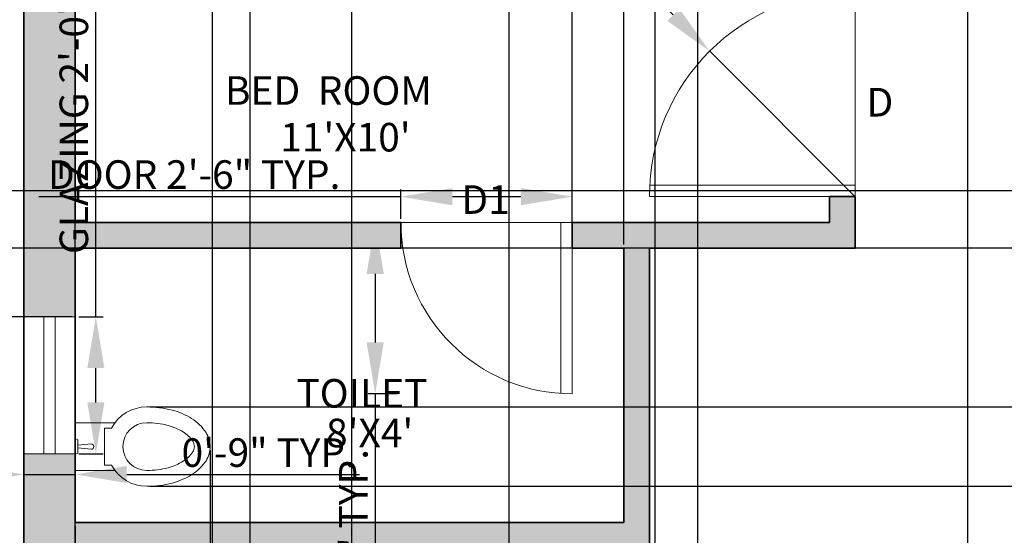
# Model space of a CAD drawing. Units: inches. Extents: x 2265 to 2807, y 1544 to 2401.
# Tile 4 of 9: x 2358 to 2531, y 2073 to 2164. Entities that reach past the tile are written whole.
import ezdxf

# ---------------------------------------------------------------- set-up
doc = ezdxf.new("R2010")
doc.units = ezdxf.units.IN
for name, color, linetype, lineweight in [('A-ANNO-DIMS', 2, 'Continuous', 18), ('A-ANNO-TEXT', 7, 'Continuous', 18), ('A-AREA-IDEN', 7, 'Continuous', 18), ('A-DOOR', 3, 'Continuous', 18), ('A-FLOR-FIXT', 8, 'Continuous', 18), ('A-GLAZ', 4, 'Continuous', 18), ('A-WALL', 7, 'Continuous', 35), ('A-WALL-PATT', 18, 'Continuous', 13)]:
    doc.layers.add(name, color=color, linetype=linetype, lineweight=lineweight)
doc.styles.add('ARIAL', font='times.ttf', dxfattribs={"height": 5})
doc.styles.get("Standard").update_dxf_attribs({"font": 'arial.ttf', "height": 5})
doc.dimstyles.new('ISO-25', dxfattribs={"dimtxt": 5, "dimasz": 9, "dimexe": 1.25, "dimexo": 0.625, "dimtad": 1, "dimlunit": 3, "dimtxsty": 'Standard', "dimcen": 2.5, "dimadec": 0, "dimazin": 0, "dimtfac": 1, "dimtmove": 0, "dimatfit": 3, "dimfxl": 1, "dimarcsym": 0})

# ---------------------------------------------------------------- blocks, each defined once
blk = doc.blocks.new('GLAZING-24IN')
for p, q in [((0, 24), (0, 0)), ((3.5, 24), (3.5, 0)), ((5.5, 24), (5.5, 0)), ((5.5, 24), (5.5, 0)), ((9, 0), (9, 24))]:
    blk.add_line(p, q)
blk = doc.blocks.new('DOOR-SWING-30IN')
for p, q in [((2, 29.93), (2, 0)), ((0, 0), (30, 0))]:
    blk.add_line(p, q)
blk.add_arc((0, 0), 30, 0, 90)
blk = doc.blocks.new('*D17')
at = {"layer": 'A-ANNO-DIMS', "color": 0, "lineweight": -2, "transparency": 16777216}
for p, q in [((2353.7, 2031.88), (2353.7, 2105.4)), ((2358.48, 2031.88), (2352.45, 2031.88)), ((2353.7, 2004.88), (2353.7, 2022.88)), ((2358.48, 1995.88), (2352.45, 1995.88))]:
    blk.add_line(p, q, dxfattribs=at)
at = {"layer": 'A-ANNO-DIMS', "color": 0, "lineweight": 100, "transparency": 16777216}
for points in [[(2352.2, 2022.88), (2355.2, 2022.88), (2353.7, 2031.88)], [(2352.2, 2004.88), (2355.2, 2004.88), (2353.7, 1995.88)]]:
    blk.add_solid(points, dxfattribs=at)
at = {"layer": 'Defpoints', "color": 0, "lineweight": 100, "transparency": 16777216}
for p in [(2353.7, 2031.88), (2359.1, 2031.88), (2359.1, 1995.88)]:
    blk.add_point(p, dxfattribs=at)
at = {"layer": 'A-ANNO-DIMS', "color": 0, "transparency": 16777216, "insert": (2350.49, 2073.14), "char_height": 5, "attachment_point": 5, "rotation": 90}
blk.add_mtext('WINDOW 3\'-0" TYP.', dxfattribs=at)
blk = doc.blocks.new('*D21')
at = {"layer": 'A-ANNO-DIMS', "color": 0, "lineweight": -2, "transparency": 16777216}
for p, q in [((2371.7, 2111.73), (2371.7, 2184.98)), ((2368.73, 2111.73), (2372.95, 2111.73)), ((2371.7, 2096.73), (2371.7, 2102.73)), ((2368.73, 2087.73), (2372.95, 2087.73))]:
    blk.add_line(p, q, dxfattribs=at)
at = {"layer": 'A-ANNO-DIMS', "color": 0, "lineweight": 100, "transparency": 16777216}
for points in [[(2370.2, 2102.73), (2373.2, 2102.73), (2371.7, 2111.73)], [(2370.2, 2096.73), (2373.2, 2096.73), (2371.7, 2087.73)]]:
    blk.add_solid(points, dxfattribs=at)
at = {"layer": 'Defpoints', "color": 0, "lineweight": 100, "transparency": 16777216}
for p in [(2368.1, 2111.73), (2371.7, 2111.73), (2368.1, 2087.73)]:
    blk.add_point(p, dxfattribs=at)
at = {"layer": 'A-ANNO-DIMS', "color": 0, "transparency": 16777216, "insert": (2368.49, 2152.86), "char_height": 5, "attachment_point": 5, "rotation": 90}
blk.add_mtext('GLAZING 2\'-0" TYP.', dxfattribs=at)
blk = doc.blocks.new('*D22')
at = {"layer": 'A-ANNO-DIMS', "color": 0, "lineweight": -2, "transparency": 16777216}
for p, q in [((2359.1, 2087.11), (2359.1, 2082.88)), ((2368.1, 2087.11), (2368.1, 2082.88)), ((2350.1, 2084.13), (2341.1, 2084.13)), ((2359.1, 2084.13), (2368.1, 2084.13)), ((2377.1, 2084.13), (2417.83, 2084.13))]:
    blk.add_line(p, q, dxfattribs=at)
at = {"layer": 'A-ANNO-DIMS', "color": 0, "lineweight": 100, "transparency": 16777216}
for points in [[(2350.1, 2085.63), (2350.1, 2082.63), (2359.1, 2084.13)], [(2377.1, 2085.63), (2377.1, 2082.63), (2368.1, 2084.13)]]:
    blk.add_solid(points, dxfattribs=at)
at = {"layer": 'Defpoints', "color": 0, "lineweight": 100, "transparency": 16777216}
for p in [(2359.1, 2087.73), (2368.1, 2087.73), (2368.1, 2084.13)]:
    blk.add_point(p, dxfattribs=at)
at = {"layer": 'A-ANNO-DIMS', "color": 0, "transparency": 16777216, "insert": (2401.96, 2087.31), "char_height": 5, "attachment_point": 5}
blk.add_mtext('0\'-9" TYP.', dxfattribs=at)
blk = doc.blocks.new('*D23')
at = {"layer": 'A-ANNO-DIMS', "color": 0, "lineweight": -2, "transparency": 16777216}
for p, q in [((2425.1, 2128.86), (2425.1, 2133.98)), ((2455.1, 2128.86), (2455.1, 2133.98)), ((2425.1, 2132.73), (2361.73, 2132.73)), ((2446.1, 2132.73), (2434.1, 2132.73))]:
    blk.add_line(p, q, dxfattribs=at)
at = {"layer": 'A-ANNO-DIMS', "color": 0, "lineweight": 100, "transparency": 16777216}
for points in [[(2434.1, 2134.23), (2434.1, 2131.23), (2425.1, 2132.73)], [(2446.1, 2134.23), (2446.1, 2131.23), (2455.1, 2132.73)]]:
    blk.add_solid(points, dxfattribs=at)
at = {"layer": 'Defpoints', "color": 0, "lineweight": 100, "transparency": 16777216}
for p in [(2425.1, 2132.73), (2425.1, 2128.23), (2455.1, 2128.23)]:
    blk.add_point(p, dxfattribs=at)
at = {"layer": 'A-ANNO-DIMS', "color": 0, "transparency": 16777216, "insert": (2388.91, 2135.95), "char_height": 5, "attachment_point": 5}
blk.add_mtext('DOOR 2\'-6" TYP.', dxfattribs=at)
blk = doc.blocks.new('*D24')
at = {"layer": 'A-ANNO-DIMS', "color": 0, "lineweight": -2, "transparency": 16777216}
for p, q in [((2424.48, 2128.23), (2419.35, 2128.23)), ((2420.6, 2119.23), (2420.6, 2107.23)), ((2424.48, 2098.23), (2419.35, 2098.23)), ((2420.6, 2098.23), (2420.6, 2057.42))]:
    blk.add_line(p, q, dxfattribs=at)
at = {"layer": 'A-ANNO-DIMS', "color": 0, "lineweight": 100, "transparency": 16777216}
for points in [[(2419.1, 2119.23), (2422.1, 2119.23), (2420.6, 2128.23)], [(2419.1, 2107.23), (2422.1, 2107.23), (2420.6, 2098.23)]]:
    blk.add_solid(points, dxfattribs=at)
at = {"layer": 'Defpoints', "color": 0, "lineweight": 100, "transparency": 16777216}
for p in [(2425.1, 2128.23), (2420.6, 2098.23), (2425.1, 2098.23)]:
    blk.add_point(p, dxfattribs=at)
at = {"layer": 'A-ANNO-DIMS', "color": 0, "transparency": 16777216, "insert": (2417.42, 2073.33), "char_height": 5, "attachment_point": 5, "rotation": 90}
blk.add_mtext('2\'-6" TYP.', dxfattribs=at)
blk = doc.blocks.new('*D40')
at = {"layer": 'A-ANNO-DIMS', "color": 0, "lineweight": -2, "transparency": 16777216}
for p, q in [((2368.1, 2005.86), (2368.1, 2297.59)), ((2392.1, 2005.86), (2392.1, 2297.59)), ((2377.1, 2296.34), (2383.1, 2296.34))]:
    blk.add_line(p, q, dxfattribs=at)
at = {"layer": 'A-ANNO-DIMS', "color": 0, "lineweight": 100, "transparency": 16777216}
for points in [[(2377.1, 2297.84), (2377.1, 2294.84), (2368.1, 2296.34)], [(2383.1, 2297.84), (2383.1, 2294.84), (2392.1, 2296.34)]]:
    blk.add_solid(points, dxfattribs=at)
at = {"layer": 'Defpoints', "color": 0, "lineweight": 100, "transparency": 16777216}
for p in [(2392.1, 2296.34), (2368.1, 2005.23), (2392.1, 2005.23)]:
    blk.add_point(p, dxfattribs=at)
at = {"layer": 'A-ANNO-DIMS', "color": 0, "transparency": 16777216, "insert": (2380.1, 2299.52), "char_height": 5, "attachment_point": 5}
blk.add_mtext('2\'-0"', dxfattribs=at)
blk = doc.blocks.new('*D43')
at = {"layer": 'A-ANNO-DIMS', "color": 0, "lineweight": -2, "transparency": 16777216}
for p, q in [((2416.49, 1959.08), (2416.49, 2297.59)), ((2444.05, 1959.08), (2444.05, 2297.59)), ((2425.49, 2296.34), (2435.05, 2296.34))]:
    blk.add_line(p, q, dxfattribs=at)
at = {"layer": 'A-ANNO-DIMS', "color": 0, "lineweight": 100, "transparency": 16777216}
for points in [[(2425.49, 2297.84), (2425.49, 2294.84), (2416.49, 2296.34)], [(2435.05, 2297.84), (2435.05, 2294.84), (2444.05, 2296.34)]]:
    blk.add_solid(points, dxfattribs=at)
at = {"layer": 'Defpoints', "color": 0, "lineweight": 100, "transparency": 16777216}
for p in [(2444.05, 2296.34), (2416.49, 1958.45), (2444.05, 1958.45)]:
    blk.add_point(p, dxfattribs=at)
at = {"layer": 'A-ANNO-DIMS', "color": 0, "transparency": 16777216, "insert": (2430.27, 2299.56), "char_height": 5, "attachment_point": 5}
blk.add_mtext('2\'-3 1/2"', dxfattribs=at)
blk = doc.blocks.new('*D45')
at = {"layer": 'A-ANNO-DIMS', "color": 0, "lineweight": -2, "transparency": 16777216}
for p, q in [((2391.72, 2088.38), (2391.72, 1546.93)), ((2368.1, 2075.11), (2368.1, 1546.93)), ((2377.1, 1548.18), (2382.72, 1548.18)), ((2391.72, 1548.18), (2430.33, 1548.18))]:
    blk.add_line(p, q, dxfattribs=at)
at = {"layer": 'A-ANNO-DIMS', "color": 0, "lineweight": 100, "transparency": 16777216}
for points in [[(2377.1, 1549.68), (2377.1, 1546.68), (2368.1, 1548.18)], [(2382.72, 1549.68), (2382.72, 1546.68), (2391.72, 1548.18)]]:
    blk.add_solid(points, dxfattribs=at)
at = {"layer": 'Defpoints', "color": 0, "lineweight": 100, "transparency": 16777216}
for p in [(2391.72, 2089), (2368.1, 2075.73), (2391.72, 1548.18)]:
    blk.add_point(p, dxfattribs=at)
at = {"layer": 'A-ANNO-DIMS', "color": 0, "transparency": 16777216, "insert": (2415.53, 1551.4), "char_height": 5, "attachment_point": 5}
blk.add_mtext('1\'-11 1/2"', dxfattribs=at)
blk = doc.blocks.new('*D46')
at = {"layer": 'A-ANNO-DIMS', "color": 0, "lineweight": -2, "transparency": 16777216}
for p, q in [((2803.21, 2104.95), (2803.21, 2128.02)), ((2381.23, 2095.95), (2804.46, 2095.95)), ((2803.21, 2082.06), (2803.21, 2095.95)), ((2381.23, 2082.06), (2804.46, 2082.06)), ((2803.21, 2073.06), (2803.21, 2064.06))]:
    blk.add_line(p, q, dxfattribs=at)
at = {"layer": 'A-ANNO-DIMS', "color": 0, "lineweight": 100, "transparency": 16777216}
for points in [[(2801.71, 2104.95), (2804.71, 2104.95), (2803.21, 2095.95)], [(2801.71, 2073.06), (2804.71, 2073.06), (2803.21, 2082.06)]]:
    blk.add_solid(points, dxfattribs=at)
at = {"layer": 'Defpoints', "color": 0, "lineweight": 100, "transparency": 16777216}
for p in [(2380.61, 2095.95), (2803.21, 2095.95), (2380.61, 2082.06)]:
    blk.add_point(p, dxfattribs=at)
at = {"layer": 'A-ANNO-DIMS', "color": 0, "transparency": 16777216, "insert": (2800.07, 2120.99), "char_height": 5, "attachment_point": 5, "rotation": 90}
blk.add_mtext('1\'-2"', dxfattribs=at)
blk = doc.blocks.new('*D47')
at = {"layer": 'A-ANNO-DIMS', "color": 0, "lineweight": -2, "transparency": 16777216}
for p, q in [((2455.1, 2124.36), (2455.1, 2297.59)), ((2464.1, 2124.36), (2464.1, 2297.59)), ((2446.1, 2296.34), (2437.1, 2296.34)), ((2455.1, 2296.34), (2464.1, 2296.34)), ((2473.1, 2296.34), (2496.64, 2296.34))]:
    blk.add_line(p, q, dxfattribs=at)
at = {"layer": 'A-ANNO-DIMS', "color": 0, "lineweight": 100, "transparency": 16777216}
for points in [[(2446.1, 2297.84), (2446.1, 2294.84), (2455.1, 2296.34)], [(2473.1, 2297.84), (2473.1, 2294.84), (2464.1, 2296.34)]]:
    blk.add_solid(points, dxfattribs=at)
at = {"layer": 'Defpoints', "color": 0, "lineweight": 100, "transparency": 16777216}
for p in [(2464.1, 2296.34), (2455.1, 2123.73), (2464.1, 2123.73)]:
    blk.add_point(p, dxfattribs=at)
at = {"layer": 'A-ANNO-DIMS', "color": 0, "transparency": 16777216, "insert": (2489.37, 2299.52), "char_height": 5, "attachment_point": 5}
blk.add_mtext('0\'-9"', dxfattribs=at)
blk = doc.blocks.new('*D49')
at = {"layer": 'A-ANNO-DIMS', "color": 0, "lineweight": -2, "transparency": 16777216}
for p, q in [((2275.29, 2132.73), (2275.29, 2155.8)), ((2367.48, 2123.73), (2274.04, 2123.73)), ((2275.29, 2111.73), (2275.29, 2123.73)), ((2367.48, 2111.73), (2274.04, 2111.73)), ((2275.29, 2102.73), (2275.29, 2093.73))]:
    blk.add_line(p, q, dxfattribs=at)
at = {"layer": 'A-ANNO-DIMS', "color": 0, "lineweight": 100, "transparency": 16777216}
for points in [[(2273.79, 2132.73), (2276.79, 2132.73), (2275.29, 2123.73)], [(2273.79, 2102.73), (2276.79, 2102.73), (2275.29, 2111.73)]]:
    blk.add_solid(points, dxfattribs=at)
at = {"layer": 'Defpoints', "color": 0, "lineweight": 100, "transparency": 16777216}
for p in [(2275.29, 2123.73), (2368.1, 2123.73), (2368.1, 2111.73)]:
    blk.add_point(p, dxfattribs=at)
at = {"layer": 'A-ANNO-DIMS', "color": 0, "transparency": 16777216, "insert": (2272.11, 2148.77), "char_height": 5, "attachment_point": 5, "rotation": 90}
blk.add_mtext('1\'-0"', dxfattribs=at)
blk = doc.blocks.new('*D50')
at = {"layer": 'A-ANNO-DIMS', "color": 0, "lineweight": -2, "transparency": 16777216}
for p, q in [((2398.67, 2169.19), (2398.67, 1546.93)), ((2469.53, 2169.19), (2469.53, 1546.93)), ((2407.67, 1548.18), (2460.53, 1548.18))]:
    blk.add_line(p, q, dxfattribs=at)
at = {"layer": 'A-ANNO-DIMS', "color": 0, "lineweight": 100, "transparency": 16777216}
for points in [[(2407.67, 1549.68), (2407.67, 1546.68), (2398.67, 1548.18)], [(2460.53, 1549.68), (2460.53, 1546.68), (2469.53, 1548.18)]]:
    blk.add_solid(points, dxfattribs=at)
at = {"layer": 'Defpoints', "color": 0, "lineweight": 100, "transparency": 16777216}
for p in [(2398.67, 2169.81), (2469.53, 2169.81), (2469.53, 1548.18)]:
    blk.add_point(p, dxfattribs=at)
at = {"layer": 'A-ANNO-DIMS', "color": 0, "transparency": 16777216, "insert": (2434.1, 1551.36), "char_height": 5, "attachment_point": 5}
blk.add_mtext('5\'-11"', dxfattribs=at)
blk = doc.blocks.new('*D60')
at = {"layer": 'A-ANNO-DIMS', "color": 0, "lineweight": -2, "transparency": 16777216}
for p, q in [((2275.29, 2142.73), (2275.29, 2151.73)), ((2580.48, 2133.73), (2274.04, 2133.73)), ((2275.29, 2133.73), (2275.29, 2123.73)), ((2580.48, 2123.73), (2274.04, 2123.73)), ((2275.29, 2114.73), (2275.29, 2087.31))]:
    blk.add_line(p, q, dxfattribs=at)
at = {"layer": 'A-ANNO-DIMS', "color": 0, "lineweight": 100, "transparency": 16777216}
for points in [[(2273.79, 2142.73), (2276.79, 2142.73), (2275.29, 2133.73)], [(2273.79, 2114.73), (2276.79, 2114.73), (2275.29, 2123.73)]]:
    blk.add_solid(points, dxfattribs=at)
at = {"layer": 'Defpoints', "color": 0, "lineweight": 100, "transparency": 16777216}
for p in [(2581.1, 2133.73), (2275.29, 2123.73), (2581.1, 2123.73)]:
    blk.add_point(p, dxfattribs=at)
at = {"layer": 'A-ANNO-DIMS', "color": 0, "transparency": 16777216, "insert": (2272.11, 2096.52), "char_height": 5, "attachment_point": 5, "rotation": 90}
blk.add_mtext('0\'-10"', dxfattribs=at)
blk = doc.blocks.new('*D63')
at = {"layer": 'A-ANNO-DIMS', "color": 0, "lineweight": -2, "transparency": 16777216}
for p, q in [((2477.1, 1993.66), (2477.1, 2297.59)), ((2524.34, 1993.66), (2524.34, 2297.59)), ((2486.1, 2296.34), (2515.34, 2296.34))]:
    blk.add_line(p, q, dxfattribs=at)
at = {"layer": 'A-ANNO-DIMS', "color": 0, "lineweight": 100, "transparency": 16777216}
for points in [[(2486.1, 2297.84), (2486.1, 2294.84), (2477.1, 2296.34)], [(2515.34, 2297.84), (2515.34, 2294.84), (2524.34, 2296.34)]]:
    blk.add_solid(points, dxfattribs=at)
at = {"layer": 'Defpoints', "color": 0, "lineweight": 100, "transparency": 16777216}
for p in [(2524.34, 2296.34), (2477.1, 1993.03), (2524.34, 1993.03)]:
    blk.add_point(p, dxfattribs=at)
at = {"layer": 'A-ANNO-DIMS', "color": 0, "transparency": 16777216, "insert": (2500.72, 2299.52), "char_height": 5, "attachment_point": 5}
blk.add_mtext('3\'-11"', dxfattribs=at)
blk = doc.blocks.new('*D66')
at = {"layer": 'A-ANNO-DIMS', "color": 0, "lineweight": -2, "transparency": 16777216}
for p, q in [((2452.75, 2184.58), (2472.78, 2164.55)), ((2504.6, 2132.73), (2479.15, 2158.19))]:
    blk.add_line(p, q, dxfattribs=at)
at = {"layer": 'A-ANNO-DIMS', "color": 0, "lineweight": 100, "transparency": 16777216}
blk.add_solid([(2473.84, 2165.61), (2471.72, 2163.49), (2479.15, 2158.19)], dxfattribs=at)
at = {"layer": 'Defpoints', "color": 0, "lineweight": 100, "transparency": 16777216}
for p in [(2479.15, 2158.19), (2504.6, 2132.73)]:
    blk.add_point(p, dxfattribs=at)
at = {"layer": 'A-ANNO-DIMS', "color": 0, "transparency": 16777216, "insert": (2461.83, 2180), "char_height": 5, "attachment_point": 5, "rotation": 315.0005}
blk.add_mtext('R3\'-0"', dxfattribs=at)

msp = doc.modelspace()

# ---------------------------------------------------------------- hatches: boundary and pattern name
at = {"layer": 'A-WALL-PATT'}
h = msp.add_hatch(color=256, dxfattribs=at)
h.dxf.hatch_style = 1
h.paths.add_polyline_path([(2416.101, 2255.733), (2359.101, 2255.733), (2359.101, 2205.483), (2368.101, 2205.483), (2368.101, 2246.733), (2416.101, 2246.733)])
h.paths.add_polyline_path([(2528.601, 2255.733), (2452.101, 2255.733), (2452.101, 2246.733), (2487.251, 2246.733), (2500.101, 2246.733), (2500.101, 2168.733), (2504.601, 2168.733), (2504.601, 2170.233), (2525.601, 2170.233), (2525.601, 2174.733), (2504.601, 2174.733), (2504.601, 2246.733), (2528.601, 2246.733)])
h.paths.add_polyline_path([(2603.601, 2255.733), (2552.601, 2255.733), (2552.601, 2246.733), (2576.601, 2246.733), (2576.601, 2174.733), (2555.601, 2174.733), (2555.601, 2170.233), (2576.601, 2170.233), (2576.601, 2123.733), (2581.101, 2123.733), (2581.101, 2246.733), (2603.601, 2246.733)])
h.paths.add_polyline_path([(2671.101, 2255.733), (2639.601, 2255.733), (2639.601, 2246.733), (2662.101, 2246.733), (2662.101, 2083.435), (2671.101, 2083.435)])
h.paths.add_polyline_path([(2671.101, 2035.435), (2662.101, 2035.435), (2662.101, 1939.233), (2644.101, 1939.233), (2644.101, 1930.233), (2662.101, 1930.233), (2662.101, 1814.733), (2644.101, 1814.733), (2644.101, 1805.733), (2671.101, 1805.733)])
h.paths.add_polyline_path([(2368.101, 1930.233), (2511.351, 1930.233), (2511.351, 1939.233), (2468.601, 1939.233), (2468.601, 2032.233), (2464.101, 2032.233), (2464.101, 1939.233), (2368.101, 1939.233), (2368.101, 1995.884), (2359.101, 1995.884), (2359.101, 1805.733), (2602.101, 1805.733), (2602.101, 1814.733), (2368.101, 1814.733)])
h.paths.add_polyline_path([(2368.101, 2071.233), (2464.101, 2071.233), (2464.101, 2062.233), (2468.601, 2062.233), (2468.601, 2123.733), (2504.601, 2123.733), (2504.601, 2132.733), (2500.101, 2132.733), (2500.101, 2128.233), (2455.101, 2128.233), (2455.101, 2123.733), (2464.101, 2123.733), (2464.101, 2075.733), (2368.101, 2075.733), (2368.101, 2087.733), (2359.101, 2087.733), (2359.101, 2031.884), (2368.101, 2031.884)])
h.paths.add_polyline_path([(2368.101, 2169.483), (2359.101, 2169.483), (2359.101, 2111.733), (2368.101, 2111.733), (2368.101, 2123.733), (2425.101, 2123.733), (2425.101, 2128.233), (2368.101, 2128.233)])

# ---------------------------------------------------------------- linework, layer by layer
at = {"layer": 'A-DOOR'}
for p, q in [((2504.601, 2132.733), (2504.601, 2168.733)), ((2468.657, 2134.733), (2504.601, 2134.733)), ((2468.601, 2132.733), (2504.601, 2132.733)), ((2455.101, 2098.233), (2455.101, 2128.233))]:
    msp.add_line(p, q, dxfattribs=at)
msp.add_arc((2504.601, 2132.733), 36, 90, 180, dxfattribs=at)
at = {"layer": 'A-FLOR-FIXT'}
for p, q in [((2368.101, 2084.834), (2368.101, 2093.172)), ((2375.049, 2093.172), (2368.101, 2093.172)), ((2373.196, 2092.245), (2373.196, 2085.761)), ((2373.196, 2092.245), (2374.462, 2092.245)), ((2368.564, 2090.161), (2368.101, 2090.392)), ((2368.564, 2087.845), (2368.564, 2090.161)), ((2368.564, 2089.235), (2370.88, 2089.466)), ((2368.101, 2087.613), (2368.564, 2087.845)), ((2370.88, 2088.54), (2368.564, 2088.771)), ((2373.196, 2085.761), (2374.462, 2085.761)), ((2375.049, 2084.834), (2368.101, 2084.834))]:
    msp.add_line(p, q, dxfattribs=at)
for centre, radius, start, end in [((2380.607, 2089.003), 6.948, 90, 152.18186), ((2380.607, 2078.226), 17.725, 75.48575, 89.99996), ((2381.983, 2083.541), 12.235, 57.99461, 75.48574), ((2380.607, 2089.003), 4.169, 90, 270), ((2380.607, 2078.226), 14.946, 75.48576, 89.99997), ((2381.983, 2083.541), 9.456, 57.9946, 75.48574), ((2384.08, 2086.896), 8.278, 33.53412, 57.99459), ((2384.08, 2086.896), 5.499, 33.53413, 57.99459), ((2387.259, 2089.003), 4.464, 0.00005, 33.53407), ((2370.88, 2089.003), 0.463, 270, 90), ((2387.259, 2089.003), 1.685, 0.00002, 33.53404), ((2387.259, 2089.003), 1.685, 326.46596, 359.99998), ((2387.259, 2089.003), 4.464, 326.46593, 359.99995), ((2384.08, 2091.11), 5.499, 302.00541, 326.46587), ((2380.607, 2089.003), 6.948, 207.81814, 270), ((2381.983, 2094.465), 9.456, 284.51426, 302.0054), ((2384.08, 2091.11), 8.278, 302.00541, 326.46588), ((2380.607, 2099.78), 14.946, 270.00003, 284.51424), ((2381.983, 2094.465), 12.235, 284.51426, 302.00539), ((2380.607, 2099.78), 17.725, 270.00004, 284.51425)]:
    msp.add_arc(centre, radius, start, end, dxfattribs=at)
at = {"layer": 'A-GLAZ'}
for p, q in [((2368.101, 2111.733), (2359.101, 2111.733)), ((2359.101, 2087.733), (2368.101, 2087.733))]:
    msp.add_line(p, q, dxfattribs=at)
at = {"layer": 'A-WALL'}
for p, q in [((2359.101, 1805.733), (2359.101, 2255.733)), ((2368.101, 2128.233), (2368.101, 2246.733)), ((2500.101, 2128.233), (2500.101, 2132.733)), ((2500.101, 2132.733), (2504.601, 2132.733)), ((2504.601, 2123.733), (2504.601, 2132.733)), ((2425.101, 2128.233), (2368.101, 2128.233)), ((2425.101, 2123.733), (2425.101, 2128.233)), ((2500.101, 2128.233), (2455.101, 2128.233)), ((2455.101, 2123.733), (2455.101, 2128.233)), ((2368.101, 2075.733), (2368.101, 2123.733)), ((2425.101, 2123.733), (2368.101, 2123.733)), ((2464.101, 2123.733), (2455.101, 2123.733)), ((2464.101, 2075.733), (2464.101, 2123.733)), ((2504.601, 2123.733), (2468.601, 2123.733)), ((2468.601, 2062.233), (2468.601, 2123.733)), ((2464.101, 2075.733), (2368.101, 2075.733))]:
    msp.add_line(p, q, dxfattribs=at)

# ---------------------------------------------------------------- block references
at = {"layer": 'A-DOOR', "rotation": 180}
msp.add_blockref('DOOR-SWING-30IN', (2455.101, 2128.233), dxfattribs=at)
at = {"layer": 'A-GLAZ'}
msp.add_blockref('GLAZING-24IN', (2359.101, 2087.733), dxfattribs=at)

# ---------------------------------------------------------------- texts
at = {"layer": 'A-ANNO-TEXT', "style": 'ARIAL'}
for s, p in [('D', (2506.604, 2146.756)), ('D1', (2435.675, 2129.726))]:
    msp.add_text(s, height=5, dxfattribs=at).set_placement(p)
at = {"layer": 'A-AREA-IDEN', "style": 'ARIAL'}
for s, p in [('BED  ROOM', (2394.289, 2148.802)), ("11'X10'", (2403.958, 2140.637)), ('TOILET', (2406.799, 2095.817)), ("  8'X4'", (2408.934, 2088.886))]:
    msp.add_text(s, height=5, dxfattribs=at).set_placement(p)

# ---------------------------------------------------------------- dimensions: what is measured, and where the dimension line sits
at = {"layer": 'A-ANNO-DIMS'}
for base, p1, p2, picture, middle in [((2444.049, 2296.343), (2416.49, 1958.452), (2444.049, 1958.452), '*D43', (2430.27, 2299.555)), ((2392.101, 2296.343), (2368.101, 2005.233), (2392.101, 2005.233), '*D40', (2380.101, 2299.521)), ((2464.101, 2296.343), (2455.101, 2123.733), (2464.101, 2123.733), '*D47', (2489.372, 2299.521)), ((2524.342, 2296.343), (2477.098, 1993.031), (2524.342, 1993.031), '*D63', (2500.72, 2299.523)), ((2469.534, 1548.185), (2398.668, 2169.812), (2469.534, 2169.812), '*D50', (2434.101, 1551.363)), ((2391.723, 1548.185), (2368.101, 2075.733), (2391.723, 2089.003), '*D45', (2415.526, 1551.395))]:
    dim = msp.add_linear_dim(base=base, p1=p1, p2=p2, dimstyle='ISO-25', override={"dimdec": 1, "dimlfac": 1, "dimrnd": 0, "dimzin": 1, "dimdsep": 46, "dimlunit": 4, "dimfrac": 2}, dxfattribs=at)
    dim.commit()
    dim.dimension.update_dxf_attribs({"geometry": picture, "text_midpoint": middle})
dim = msp.add_radius_dim(center=(2504.601, 2132.733), mpoint=(2479.145, 2158.189), dimstyle='ISO-25', override={"dimdec": 1, "dimlfac": 1, "dimrnd": 0, "dimzin": 1, "dimdsep": 46, "dimlunit": 4, "dimfrac": 2}, dxfattribs=at)
dim.commit()
dim.dimension.update_dxf_attribs({"geometry": '*D66', "text_midpoint": (2461.832, 2179.998)})
for base, p1, p2, angle, text, picture, middle in [((2371.701, 2111.733), (2368.101, 2087.733), (2368.101, 2111.733), 90, 'GLAZING <> TYP.', '*D21', (2368.491, 2152.857)), ((2425.101, 2132.733), (2455.101, 2128.233), (2425.101, 2128.233), 180, 'DOOR <> TYP.', '*D23', (2388.914, 2135.945)), ((2420.601, 2098.233), (2425.101, 2128.233), (2425.101, 2098.233), 270, '<> TYP.', '*D24', (2417.423, 2073.327)), ((2353.701, 2031.884), (2359.101, 1995.884), (2359.101, 2031.884), 90, 'WINDOW <> TYP.', '*D17', (2350.488, 2073.144))]:
    dim = msp.add_linear_dim(base=base, p1=p1, p2=p2, angle=angle, text=text, dimstyle='ISO-25', override={"dimdec": 1, "dimlfac": 1, "dimrnd": 0, "dimzin": 1, "dimdsep": 46, "dimlunit": 4, "dimfrac": 2}, dxfattribs=at)
    dim.commit()
    dim.dimension.update_dxf_attribs({"geometry": picture, "text_midpoint": middle})
for base, p1, p2, picture, middle in [((2275.289, 2123.733), (2368.101, 2111.733), (2368.101, 2123.733), '*D49', (2272.111, 2148.769)), ((2275.289, 2123.733), (2581.101, 2133.733), (2581.101, 2123.733), '*D60', (2272.111, 2096.52)), ((2803.21, 2095.951), (2380.607, 2082.055), (2380.607, 2095.951), '*D46', (2800.075, 2120.986))]:
    dim = msp.add_linear_dim(base=base, p1=p1, p2=p2, angle=90, dimstyle='ISO-25', override={"dimdec": 1, "dimlfac": 1, "dimrnd": 0, "dimzin": 1, "dimdsep": 46, "dimlunit": 4, "dimfrac": 2}, dxfattribs=at)
    dim.commit()
    dim.dimension.update_dxf_attribs({"geometry": picture, "text_midpoint": middle})
dim = msp.add_linear_dim(base=(2368.101, 2084.133), p1=(2359.101, 2087.733), p2=(2368.101, 2087.733), text='<> TYP.', dimstyle='ISO-25', override={"dimdec": 1, "dimlfac": 1, "dimrnd": 0, "dimzin": 1, "dimdsep": 46, "dimlunit": 4, "dimfrac": 2}, dxfattribs=at)
dim.commit()
dim.dimension.update_dxf_attribs({"geometry": '*D22', "text_midpoint": (2401.965, 2087.311)})

doc.saveas('drawing.dxf')
